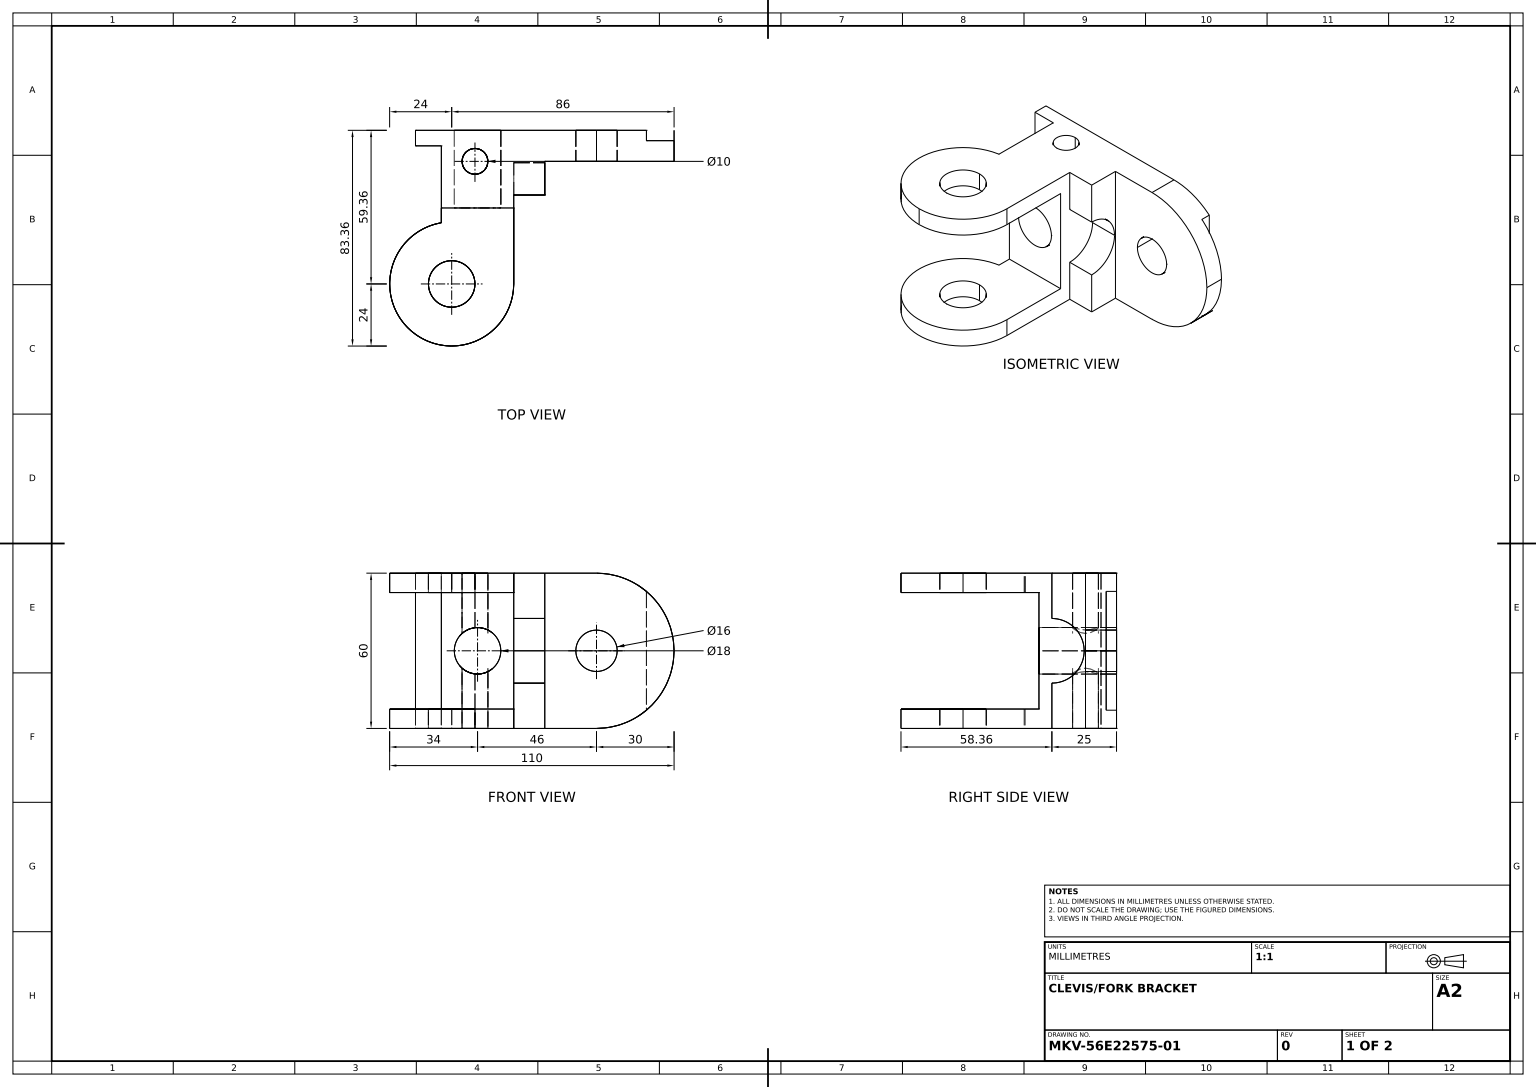
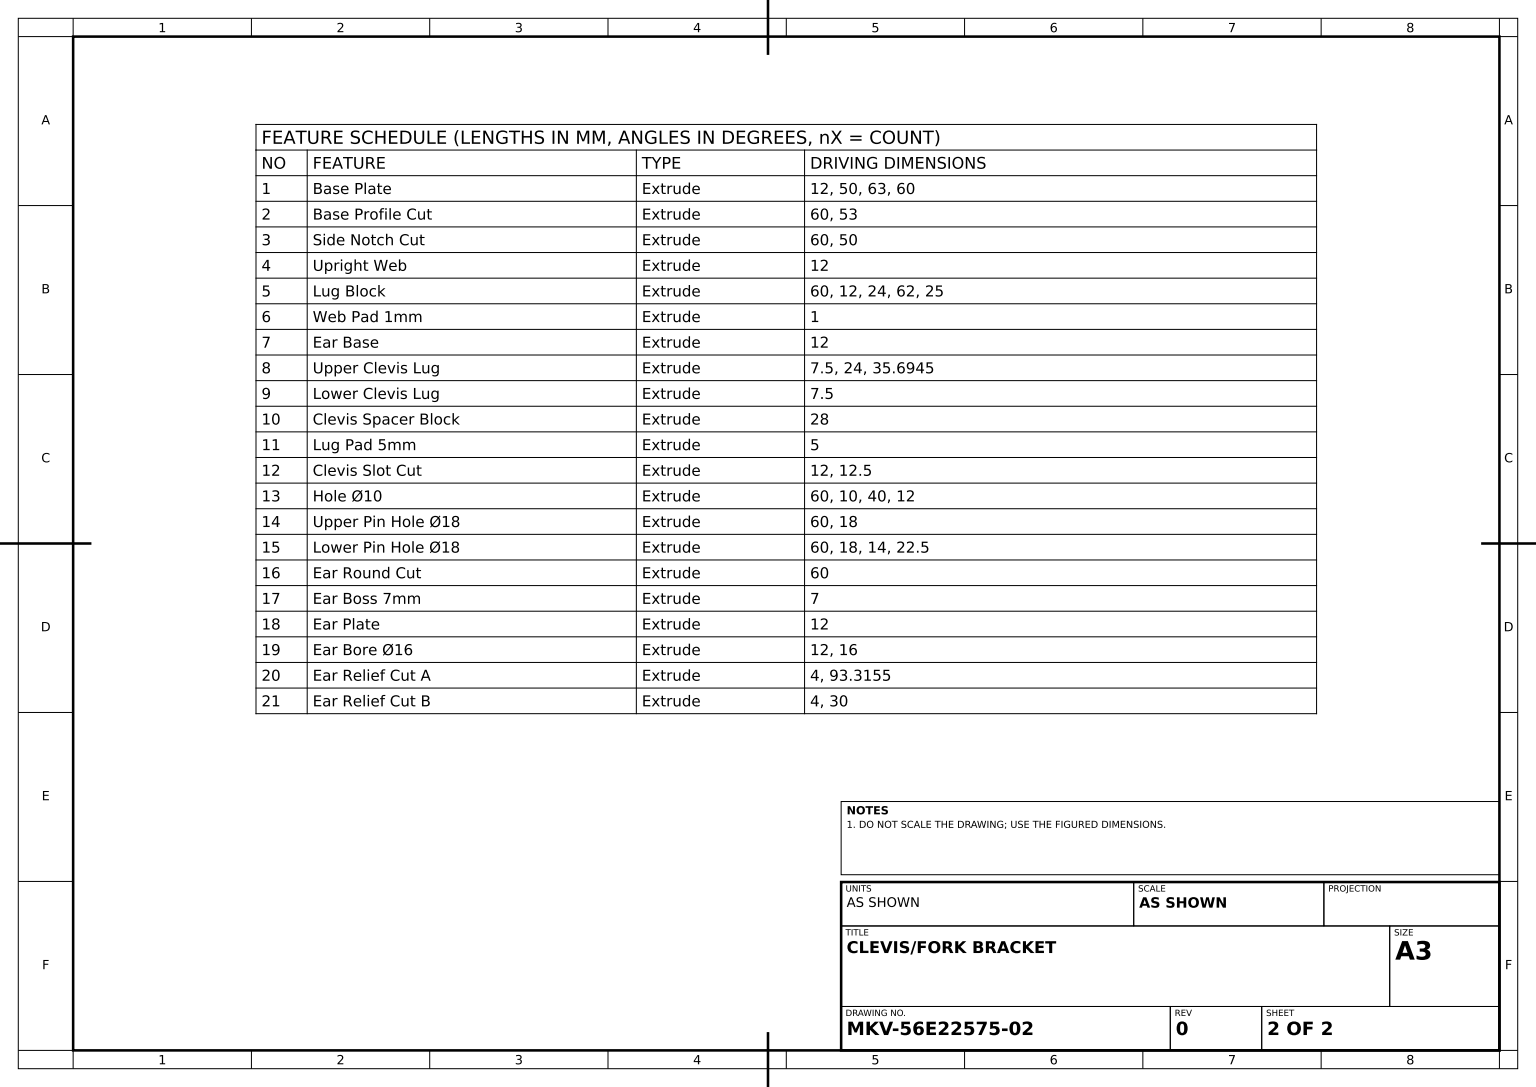
SolidWorks part; units mm, degrees
material "Plain Carbon Steel"
ref_plane "Front Plane" through (0, 0, 0) normal (0, 0, 1) x (1, 0, 0)
ref_plane "Top Plane" through (0, 0, 0) normal (0, 1, 0) x (1, 0, 0)
ref_plane "Right Plane" through (0, 0, 0) normal (1, 0, 0) x (0, 0, -1)
sketch "Base Plate Sketch" plane through (0, 0, 0) normal (0, 0, 1) x (1, 0, 0)
  line L0 (0, 0) -> (50, 0)
  line L2 (50, 60) -> (0, 60)
  line L3 (0, 60) -> (0, 0)
  line L4 (50, 0) -> (63, 0)
  line L5 (63, 0) -> (63, 60)
  line L6 (63, 60) -> (50, 60)
  dimension "D1" = 50
  dimension "D2" = 63
  dimension "D3" = 60
extrude "Base Plate" add sketch "Base Plate Sketch" along normal blind 12
sketch "Base Profile Cut Sketch" plane through (0, 0, 0) normal (0, -1, 0) x (1, 0, 0)
  line L0 (0, 0) -> (0, 6)
  line L1 (63, 12) -> (63, 0) construction
  line L2 (0, 12) -> (0, 0) construction
  line L3 (0, 6) -> (10, 6)
  line L4 (10, 6) -> (10, 12)
  line L5 (0, 12) -> (63, 12) construction
  line L6 (10, 12) -> (0, 12)
  line L7 (0, 12) -> (0, 6)
  line M3 (63, 12) -> (0, 12)
  line M4 (0, 12) -> (0, 0)
  dimension "D1" = 53
extrude "Base Profile Cut" cut sketch "Base Profile Cut Sketch" against normal blind 60 contours L3 L4 M3 M4
sketch "Side Notch Sketch" plane through (0, 0, 0) normal (0, -1, 0) x (1, 0, 0)
  line L0 (0, 6) -> (0, 0) construction
  line L1 (0, 0) -> (63, 0) construction
  line L2 (50, 0) -> (50, 12)
  line L3 (10, 12) -> (63, 12) construction
  line L4 (50, 12) -> (63, 12)
  line L5 (63, 12) -> (63, 0)
  line L6 (63, 12) -> (63, 0) construction
  line L7 (63, 0) -> (50, 0)
  dimension "D1" = 50
extrude "Side Notch Cut" cut sketch "Side Notch Sketch" against normal blind 60
sketch "Upright Web Sketch" plane through (0, 0, 12) normal (0, 0, 1) x (1, 0, 0)
  line L0 (50, 60) -> (62, 60)
  line L1 (62, 60) -> (62, 0)
  line L2 (62, 0) -> (50, 0)
  line L3 (50, 0) -> (50, 60)
  line L4 (50, 60) -> (50, 0) construction
  dimension "D1" = 12
extrude "Upright Web" add sketch "Upright Web Sketch" against normal blind 12
sketch "Lug Block Sketch" plane through (0, 0, 0) normal (0, -1, 0) x (1, 0, 0)
  line L0 (0, 12) -> (50, 12)
  line L1 (50, 12) -> (50, 25)
  line L2 (50, 25) -> (38, 25)
  line L3 (38, 25) -> (38, 12)
  line L4 (62, 0) -> (62, 12) construction
  line L5 (0, 0) -> (62, 0) construction
  line M3 (62, 12) -> (10, 12)
  dimension "D1" = 12
  dimension "D2" = 24
  dimension "D3" = 62
  dimension "D4" = 25
extrude "Lug Block" add sketch "Lug Block Sketch" against normal blind 60 contours L2 L3 L1 M3
sketch "Web Pad Sketch" plane through (62, 0, 0) normal (1, 0, 0) x (0, 0, -1)
  line L0 (-12, 60) -> (0, 60)
  line L1 (0, 60) -> (0, 0)
  line L2 (0, 0) -> (-12, 0)
  line L3 (-12, 0) -> (-12, 60)
extrude "Web Pad 1mm" add sketch "Web Pad Sketch" along normal blind 1
sketch "Ear Base Sketch" plane through (0, 0, 12) normal (0, 0, 1) x (1, 0, 0)
  line L0 (63, 60) -> (63, 0) construction
  line L1 (63, 60) -> (63, 0)
  arc A0 (63, 0) -> (63, 60) centre (63, 30) ccw
  dimension "D1" = 60
extrude "Ear Base" add sketch "Ear Base Sketch" against normal blind 12
sketch "Upper Clevis Lug Sketch" plane through (0, 0, 0) normal (0, -1, 0) x (1, 0, 0)
  line L0 (10, 12) -> (38, 12)
  line L1 (10, 12) -> (10, 35.6945)
  line L3 (38, 59.3588) -> (38, 25)
  line L4 (0, 0) -> (63, 0) construction
  line L13 (0, 0) -> (63, 0)
  line L14 (63, 0) -> (63, 12)
  line L15 (63, 12) -> (50, 12)
  line L16 (50, 12) -> (50, 25)
  line L17 (50, 25) -> (38, 25)
  line L18 (38, 25) -> (38, 12)
  line L19 (38, 12) -> (10, 12)
  line L20 (10, 12) -> (10, 6)
  line L21 (10, 6) -> (0, 6)
  line L22 (0, 6) -> (0, 0)
  line L23 (0, 0) -> (63, 0)
  line L24 (63, 0) -> (63, 12)
  line L25 (63, 12) -> (50, 12)
  line L26 (50, 12) -> (50, 25)
  line L27 (50, 25) -> (38, 25)
  line L29 (38, 12) -> (10, 12)
  line L30 (10, 12) -> (10, 6)
  line L31 (10, 6) -> (0, 6)
  line L32 (0, 6) -> (0, 0)
  arc A0 (38, 59.3588) -> (10, 35.6945) centre (14, 59.3588) ccw
  line M16 (38, 25) -> (38, 12)
  line M17 (38, 12) -> (10, 12)
  dimension "D1" = 48
  dimension "D3" = 24
  dimension "D2" = 0
  dimension "D4" = 35.6945
extrude "Upper Clevis Lug" add sketch "Upper Clevis Lug Sketch" against normal blind 7.5 contours L3 A0 L1 M17 M16
sketch "Lower Clevis Lug Sketch" plane through (0, 60, 0) normal (0, 1, 0) x (1, 0, 0)
  line L0 (38, -12) -> (38, -59.3588)
  line L1 (10, -12) -> (10, -35.6945)
  line L2 (38, -12) -> (10, -12)
  arc A0 (10, -35.6945) -> (38, -59.3588) centre (14, -59.3588) ccw
  dimension "D1" = 48
extrude "Lower Clevis Lug" add sketch "Lower Clevis Lug Sketch" against normal blind 7.5
sketch "Clevis Spacer Sketch" plane through (38, 0, 0) normal (-1, 0, 0) x (0, 0, 1)
  line L0 (12, 52.5) -> (25, 52.5)
  line L1 (25, 52.5) -> (25, 7.5)
  line L2 (25, 7.5) -> (12, 7.5)
  line L3 (12, 7.5) -> (12, 52.5)
extrude "Clevis Spacer Block" add sketch "Clevis Spacer Sketch" along normal blind 28
sketch "Lug Pad Sketch" plane through (0, 0, 25) normal (0, 0, 1) x (1, 0, 0)
  line L0 (10, 52.5) -> (38, 52.5)
  line L1 (38, 52.5) -> (38, 7.5)
  line L2 (10, 7.5) -> (38, 7.5) construction
  line L3 (38, 7.5) -> (-10, 7.5) construction
  line L4 (38, 7.5) -> (10, 7.5)
  line L5 (10, 60) -> (10, 0) construction
  line L6 (10, 7.5) -> (10, 52.5)
extrude "Lug Pad 5mm" add sketch "Lug Pad Sketch" along normal blind 5
sketch "Clevis Slot Sketch" plane through (50, 0, 0) normal (1, 0, 0) x (0, 0, -1)
  line L0 (-25, 60) -> (-25, 0) construction
  line L1 (-25, 42.5) -> (-25, 17.5)
  arc A0 (-25, 17.5) -> (-25, 42.5) centre (-25, 30) ccw
  dimension "D1" = 25
  dimension "D2" = 12.5
extrude "Clevis Slot Cut" cut sketch "Clevis Slot Sketch" against normal blind 12
sketch "Hole Ø10 Sketch" plane through (0, 0, 0) normal (0, -1, 0) x (1, 0, 0)
  line L0 (63, 12) -> (63, 0) construction
  line L1 (0, 0) -> (63, 0) construction
  circle A0 centre (23, 12) radius 5
  dimension "D1" = 10
  dimension "D2" = 10
  dimension "D3" = 40
  dimension "D4" = 12
extrude "Hole Ø10" cut sketch "Hole Ø10 Sketch" against normal blind 60
sketch "Upper Pin Hole Ø18 Sketch" plane through (0, 0, 0) normal (0, -1, 0) x (1, 0, 0)
  circle A0 centre (14, 59.3588) radius 9
  dimension "D1" = 18
  dimension "D2" = 18
extrude "Upper Pin Hole Ø18" cut sketch "Upper Pin Hole Ø18 Sketch" against normal blind 60
sketch "Lower Pin Hole Ø18 Sketch" plane through (0, 0, 30) normal (0, 0, 1) x (1, 0, 0)
  line L0 (10, 52.5) -> (10, 7.5) construction
  line L1 (10, 7.5) -> (38, 7.5) construction
  circle A0 centre (24, 30) radius 9
  dimension "D1" = 18
  dimension "D2" = 18
  dimension "D3" = 14
  dimension "D4" = 22.5
extrude "Lower Pin Hole Ø18" cut sketch "Lower Pin Hole Ø18 Sketch" against normal blind 60
sketch "Ear Round Cut Sketch" plane through (0, 0, 12) normal (0, 0, 1) x (1, 0, 0)
  line L0 (63, 60) -> (63, 0)
  arc A0 (63, 0) -> (63, 60) centre (63, 30) ccw
  dimension "D1" = 60
extrude "Ear Round Cut" cut sketch "Ear Round Cut Sketch" against normal blind 60
sketch "Ear Boss Sketch" plane through (63, 0, 0) normal (1, 0, 0) x (0, 0, -1)
  line L0 (-12, 60) -> (0, 60)
  line L1 (0, 60) -> (0, 0)
  line L2 (0, 0) -> (-12, 0)
  line L3 (-12, 0) -> (-12, 60)
extrude "Ear Boss 7mm" add sketch "Ear Boss Sketch" along normal blind 7
sketch "Ear Plate Sketch" plane through (0, 0, 12) normal (0, 0, 1) x (1, 0, 0)
  line L0 (70, 60) -> (70, 0) construction
  line L1 (70, 60) -> (70, 0)
  arc A0 (70, 0) -> (70, 60) centre (70, 30) ccw
  dimension "D1" = 60
extrude "Ear Plate" add sketch "Ear Plate Sketch" against normal blind 12
sketch "Ear Bore Ø16 Sketch" plane through (0, 0, 12) normal (0, 0, 1) x (1, 0, 0)
  circle A0 centre (70, 30) radius 8
  dimension "D1" = 16
  dimension "D2" = 16
extrude "Ear Bore Ø16" cut sketch "Ear Bore Ø16 Sketch" against normal blind 12
sketch "Ear Relief A Sketch" plane through (0, 0, 0) normal (0, 0, -1) x (-1, 0, 0)
  line L0 (-93.3155, 48.8783) -> (-93.3155, 11.1217)
  arc A0 (-70, 60) -> (-70, 0) centre (-70, 30) ccw construction
  arc A1 (-93.3155, 48.8783) -> (-93.3155, 11.1217) centre (-70, 30) ccw
  dimension "D1" = 60
  dimension "D2" = 93.3155
extrude "Ear Relief Cut A" cut sketch "Ear Relief A Sketch" against normal blind 4
sketch "Ear Relief B Sketch" plane through (0, 0, 0) normal (0, 0, -1) x (-1, 0, 0)
  line L0 (-93.3155, 11.1217) -> (-93.3155, 48.8783) construction
  line L2 (-89.3155, 30) -> (-89.3155, 52.9546)
  line L3 (-89.3155, 52.9546) -> (-89.3155, 7.0454)
  arc A0 (-89.3155, 52.9546) -> (-89.3155, 7.0454) centre (-70, 30) ccw
  arc M3 (-70, 60) -> (-93.3155, 48.8783) centre (-70, 30) ccw
  line M4 (-93.3155, 48.8783) -> (-93.3155, 11.1217)
  arc M5 (-93.3155, 11.1217) -> (-70, 0) centre (-70, 30) ccw
  dimension "D1" = 60
  dimension "D2" = 30
  dimension "D3" = 4
extrude "Ear Relief Cut B" cut sketch "Ear Relief B Sketch" against normal blind 4 contours L3 L2 M3 M4 M5
